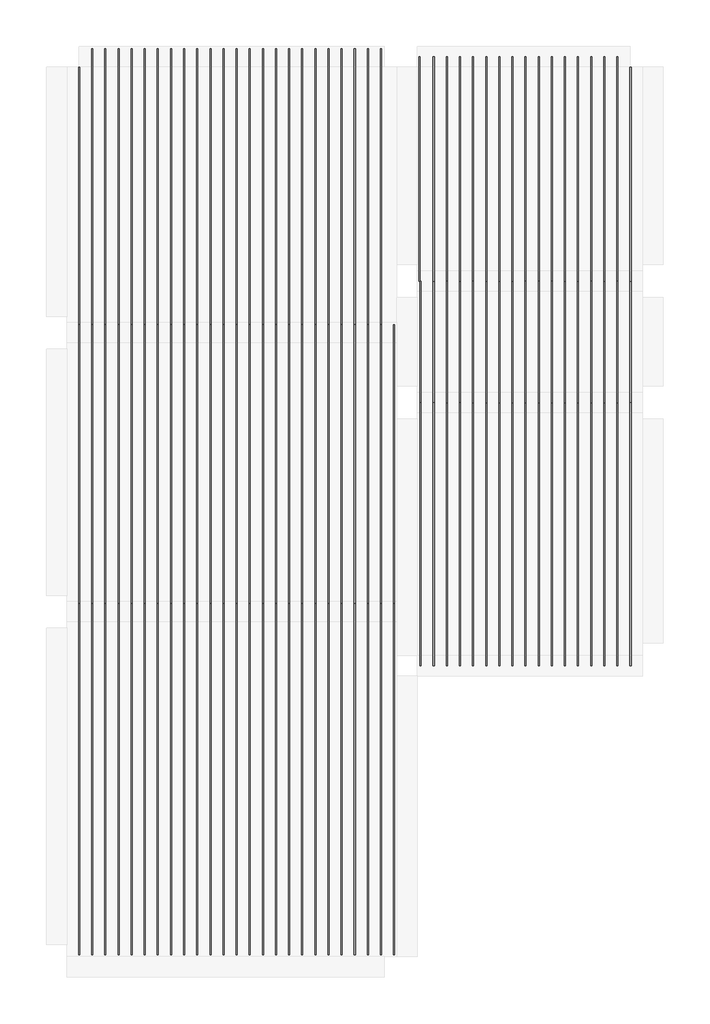
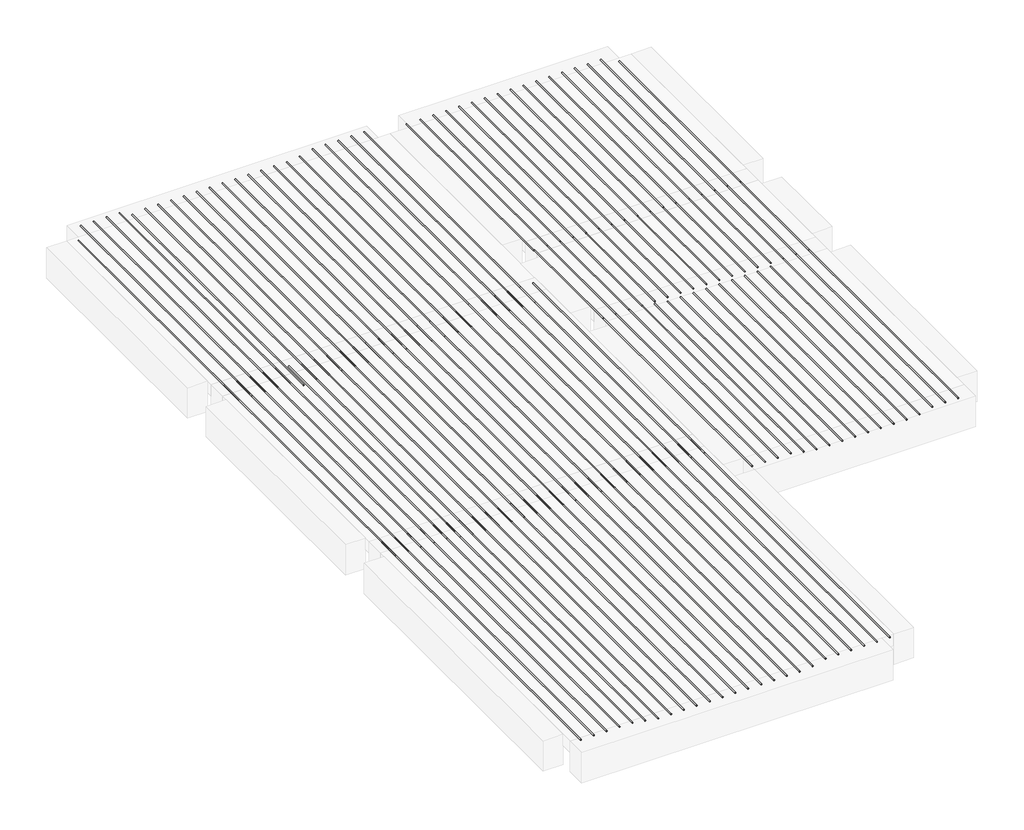
# One storey, part 2 of 2: 125 reinforcing bars.
"""IFC4 building model written with IfcOpenShell, lengths in millimetres."""

from ifc_helpers import new_model, si_unit, origin, place, context, project, spatial, polyline, segment, composite_curve, element, save
from ifc_brep_helpers import swept_disk

model = new_model("IFC4")

# Units and contexts
model_context = context("Model", 3, world=origin())
ifc_project = project(units=[si_unit("LENGTHUNIT", "METRE", prefix="MILLI")], contexts=[model_context])

# Site, building, storey
site = spatial("IfcSite", under=ifc_project)
building = spatial("IfcBuilding", under=site)
storey = spatial("IfcBuildingStorey", under=building, Elevation=0.0)

# Reinforcing bars
placement = place(None, origin())
element("IfcReinforcingBar", 1, at=placement, inside=storey, context=model_context, shape_type="SolidModel", body=[
    swept_disk(composite_curve([segment(polyline([(-8027.4883428, -144.0769256, -45.3573217), (-8027.4883428, 4206.4668244, -45.3573217)]), True, "CONTINUOUS")], self_intersect=False), 6.35),
])
element("IfcReinforcingBar", 2, at=placement, inside=storey, context=model_context, shape_type="SolidModel", body=[
    swept_disk(composite_curve([segment(polyline([(-8190.1883428, -144.0769256, -45.3573217), (-8190.1883428, 4206.4668244, -45.3573217)]), True, "CONTINUOUS")], self_intersect=False), 6.35),
])
element("IfcReinforcingBar", 3, at=placement, inside=storey, context=model_context, shape_type="SolidModel", body=[
    swept_disk(composite_curve([segment(polyline([(-8352.8883428, -144.0769256, -45.3573217), (-8352.8883428, 4206.4668244, -45.3573217)]), True, "CONTINUOUS")], self_intersect=False), 6.35),
])
element("IfcReinforcingBar", 4, at=placement, inside=storey, context=model_context, shape_type="SolidModel", body=[
    swept_disk(composite_curve([segment(polyline([(-8515.5883428, -144.0769256, -45.3573217), (-8515.5883428, 4206.4668244, -45.3573217)]), True, "CONTINUOUS")], self_intersect=False), 6.35),
])
element("IfcReinforcingBar", 5, at=placement, inside=storey, context=model_context, shape_type="SolidModel", body=[
    swept_disk(composite_curve([segment(polyline([(-8678.2883428, -144.0769256, -45.3573217), (-8678.2883428, 4206.4668244, -45.3573217)]), True, "CONTINUOUS")], self_intersect=False), 6.35),
])
element("IfcReinforcingBar", 6, at=placement, inside=storey, context=model_context, shape_type="SolidModel", body=[
    swept_disk(composite_curve([segment(polyline([(-8840.9883428, -144.0769256, -45.3573217), (-8840.9883428, 4206.4668244, -45.3573217)]), True, "CONTINUOUS")], self_intersect=False), 6.35),
])
element("IfcReinforcingBar", 7, at=placement, inside=storey, context=model_context, shape_type="SolidModel", body=[
    swept_disk(composite_curve([segment(polyline([(-9003.6883428, -144.0769256, -87.8573217), (-9003.6883428, 4206.4668244, -87.8573217)]), True, "CONTINUOUS")], self_intersect=False), 6.35),
])
element("IfcReinforcingBar", 8, at=placement, inside=storey, context=model_context, shape_type="SolidModel", body=[
    swept_disk(composite_curve([segment(polyline([(-11118.7883428, -144.0769256, -75.3573217), (-11118.7883428, 4206.4668244, -75.3573217)]), True, "CONTINUOUS")], self_intersect=False), 6.35),
])
element("IfcReinforcingBar", 9, at=placement, inside=storey, context=model_context, shape_type="SolidModel", body=[
    swept_disk(composite_curve([segment(polyline([(-11281.4883428, -144.0769256, -45.3573217), (-11281.4883428, 4206.4668244, -45.3573217)]), True, "CONTINUOUS")], self_intersect=False), 6.35),
])
element("IfcReinforcingBar", 10, at=placement, inside=storey, context=model_context, shape_type="SolidModel", body=[
    swept_disk(composite_curve([segment(polyline([(-11444.1883428, -144.0769256, -45.3573217), (-11444.1883428, 4206.4668244, -45.3573217)]), True, "CONTINUOUS")], self_intersect=False), 6.35),
])
element("IfcReinforcingBar", 11, at=placement, inside=storey, context=model_context, shape_type="SolidModel", body=[
    swept_disk(composite_curve([segment(polyline([(-11606.8883428, -144.0769256, -45.3573217), (-11606.8883428, 4206.4668244, -45.3573217)]), True, "CONTINUOUS")], self_intersect=False), 6.35),
])
element("IfcReinforcingBar", 12, at=placement, inside=storey, context=model_context, shape_type="SolidModel", body=[
    swept_disk(composite_curve([segment(polyline([(-11769.5883428, -144.0769256, -45.3573217), (-11769.5883428, 4206.4668244, -45.3573217)]), True, "CONTINUOUS")], self_intersect=False), 6.35),
])
element("IfcReinforcingBar", 13, at=placement, inside=storey, context=model_context, shape_type="SolidModel", body=[
    swept_disk(composite_curve([segment(polyline([(-11932.2883428, -144.0769256, -45.3573217), (-11932.2883428, 4206.4668244, -45.3573217)]), True, "CONTINUOUS")], self_intersect=False), 6.35),
])
element("IfcReinforcingBar", 14, at=placement, inside=storey, context=model_context, shape_type="SolidModel", body=[
    swept_disk(composite_curve([segment(polyline([(-9166.3883428, -144.0769256, -104.3861355), (-9166.3883428, 4206.4668244, -104.3861355)]), True, "CONTINUOUS")], self_intersect=False), 6.35),
])
element("IfcReinforcingBar", 15, at=placement, inside=storey, context=model_context, shape_type="SolidModel", body=[
    swept_disk(composite_curve([segment(polyline([(-9329.0883428, -144.0769256, -104.3861355), (-9329.0883428, 4206.4668244, -104.3861355)]), True, "CONTINUOUS")], self_intersect=False), 6.35),
])
element("IfcReinforcingBar", 16, at=placement, inside=storey, context=model_context, shape_type="SolidModel", body=[
    swept_disk(composite_curve([segment(polyline([(-9491.7883428, -144.0769256, -104.3861355), (-9491.7883428, 4206.4668244, -104.3861355)]), True, "CONTINUOUS")], self_intersect=False), 6.35),
])
element("IfcReinforcingBar", 17, at=placement, inside=storey, context=model_context, shape_type="SolidModel", body=[
    swept_disk(composite_curve([segment(polyline([(-9654.4883428, -144.0769256, -104.3861355), (-9654.4883428, 4206.4668244, -104.3861355)]), True, "CONTINUOUS")], self_intersect=False), 6.35),
])
element("IfcReinforcingBar", 18, at=placement, inside=storey, context=model_context, shape_type="SolidModel", body=[
    swept_disk(composite_curve([segment(polyline([(-9817.1883428, -144.0769256, -104.3861355), (-9817.1883428, 4206.4668244, -104.3861355)]), True, "CONTINUOUS")], self_intersect=False), 6.35),
])
element("IfcReinforcingBar", 19, at=placement, inside=storey, context=model_context, shape_type="SolidModel", body=[
    swept_disk(composite_curve([segment(polyline([(-9979.8883428, -144.0769256, -104.3861355), (-9979.8883428, 4206.4668244, -104.3861355)]), True, "CONTINUOUS")], self_intersect=False), 6.35),
])
element("IfcReinforcingBar", 20, at=placement, inside=storey, context=model_context, shape_type="SolidModel", body=[
    swept_disk(composite_curve([segment(polyline([(-10142.5883428, -144.0769256, -104.3861355), (-10142.5883428, 4206.4668244, -104.3861355)]), True, "CONTINUOUS")], self_intersect=False), 6.35),
])
element("IfcReinforcingBar", 21, at=placement, inside=storey, context=model_context, shape_type="SolidModel", body=[
    swept_disk(composite_curve([segment(polyline([(-10305.2883428, -144.0769256, -104.3861355), (-10305.2883428, 4206.4668244, -104.3861355)]), True, "CONTINUOUS")], self_intersect=False), 6.35),
])
element("IfcReinforcingBar", 22, at=placement, inside=storey, context=model_context, shape_type="SolidModel", body=[
    swept_disk(composite_curve([segment(polyline([(-10467.9883428, -144.0769256, -104.3861355), (-10467.9883428, 4206.4668244, -104.3861355)]), True, "CONTINUOUS")], self_intersect=False), 6.35),
])
element("IfcReinforcingBar", 23, at=placement, inside=storey, context=model_context, shape_type="SolidModel", body=[
    swept_disk(composite_curve([segment(polyline([(-10630.6883428, -144.0769256, -104.3861355), (-10630.6883428, 4206.4668244, -104.3861355)]), True, "CONTINUOUS")], self_intersect=False), 6.35),
])
element("IfcReinforcingBar", 24, at=placement, inside=storey, context=model_context, shape_type="SolidModel", body=[
    swept_disk(composite_curve([segment(polyline([(-10793.3883428, -144.0769256, -104.3861355), (-10793.3883428, 4206.4668244, -104.3861355)]), True, "CONTINUOUS")], self_intersect=False), 6.35),
])
element("IfcReinforcingBar", 25, at=placement, inside=storey, context=model_context, shape_type="SolidModel", body=[
    swept_disk(composite_curve([segment(polyline([(-10956.0883428, -144.0769256, -104.3861355), (-10956.0883428, 4206.4668244, -104.3861355)]), True, "CONTINUOUS")], self_intersect=False), 6.35),
])
element("IfcReinforcingBar", 26, at=placement, inside=storey, context=model_context, shape_type="SolidModel", body=[
    swept_disk(composite_curve([segment(polyline([(-8027.4883428, 3911.5030538, -45.3573217), (-8027.4883428, 7660.8668244, -45.3573217)]), True, "CONTINUOUS")], self_intersect=False), 6.35),
])
element("IfcReinforcingBar", 27, at=placement, inside=storey, context=model_context, shape_type="SolidModel", body=[
    swept_disk(composite_curve([segment(polyline([(-8190.1883428, 3911.5030538, -45.3573217), (-8190.1883428, 7660.8668244, -45.3573217)]), True, "CONTINUOUS")], self_intersect=False), 6.35),
])
element("IfcReinforcingBar", 28, at=placement, inside=storey, context=model_context, shape_type="SolidModel", body=[
    swept_disk(composite_curve([segment(polyline([(-8352.8883428, 3911.5030538, -45.3573217), (-8352.8883428, 7660.8668244, -45.3573217)]), True, "CONTINUOUS")], self_intersect=False), 6.35),
])
element("IfcReinforcingBar", 29, at=placement, inside=storey, context=model_context, shape_type="SolidModel", body=[
    swept_disk(composite_curve([segment(polyline([(-8515.5883428, 3911.5030538, -45.3573217), (-8515.5883428, 7660.8668244, -45.3573217)]), True, "CONTINUOUS")], self_intersect=False), 6.35),
])
element("IfcReinforcingBar", 30, at=placement, inside=storey, context=model_context, shape_type="SolidModel", body=[
    swept_disk(composite_curve([segment(polyline([(-8678.2883428, 3911.5030538, -45.3573217), (-8678.2883428, 7660.8668244, -45.3573217)]), True, "CONTINUOUS")], self_intersect=False), 6.35),
])
element("IfcReinforcingBar", 31, at=placement, inside=storey, context=model_context, shape_type="SolidModel", body=[
    swept_disk(composite_curve([segment(polyline([(-8840.9883428, 3911.5030538, -45.3573217), (-8840.9883428, 7660.8668244, -45.3573217)]), True, "CONTINUOUS")], self_intersect=False), 6.35),
])
element("IfcReinforcingBar", 32, at=placement, inside=storey, context=model_context, shape_type="SolidModel", body=[
    swept_disk(composite_curve([segment(polyline([(-9003.6883428, 3911.5030538, -87.8573217), (-9003.6883428, 7660.8668244, -87.8573217)]), True, "CONTINUOUS")], self_intersect=False), 6.35),
])
element("IfcReinforcingBar", 33, at=placement, inside=storey, context=model_context, shape_type="SolidModel", body=[
    swept_disk(composite_curve([segment(polyline([(-11118.7883428, 3911.5030538, -75.3573217), (-11118.7883428, 7660.8668244, -75.3573217)]), True, "CONTINUOUS")], self_intersect=False), 6.35),
])
element("IfcReinforcingBar", 34, at=placement, inside=storey, context=model_context, shape_type="SolidModel", body=[
    swept_disk(composite_curve([segment(polyline([(-11281.4883428, 3911.5030538, -45.3573217), (-11281.4883428, 7660.8668244, -45.3573217)]), True, "CONTINUOUS")], self_intersect=False), 6.35),
])
element("IfcReinforcingBar", 35, at=placement, inside=storey, context=model_context, shape_type="SolidModel", body=[
    swept_disk(composite_curve([segment(polyline([(-11444.1883428, 3911.5030538, -45.3573217), (-11444.1883428, 7660.8668244, -45.3573217)]), True, "CONTINUOUS")], self_intersect=False), 6.35),
])
element("IfcReinforcingBar", 36, at=placement, inside=storey, context=model_context, shape_type="SolidModel", body=[
    swept_disk(composite_curve([segment(polyline([(-11606.8883428, 3911.5030538, -45.3573217), (-11606.8883428, 7660.8668244, -45.3573217)]), True, "CONTINUOUS")], self_intersect=False), 6.35),
])
element("IfcReinforcingBar", 37, at=placement, inside=storey, context=model_context, shape_type="SolidModel", body=[
    swept_disk(composite_curve([segment(polyline([(-11769.5883428, 3911.5030538, -45.3573217), (-11769.5883428, 7660.8668244, -45.3573217)]), True, "CONTINUOUS")], self_intersect=False), 6.35),
])
element("IfcReinforcingBar", 38, at=placement, inside=storey, context=model_context, shape_type="SolidModel", body=[
    swept_disk(composite_curve([segment(polyline([(-11932.2883428, 3911.5030538, -45.3573217), (-11932.2883428, 7660.8668244, -45.3573217)]), True, "CONTINUOUS")], self_intersect=False), 6.35),
])
element("IfcReinforcingBar", 39, at=placement, inside=storey, context=model_context, shape_type="SolidModel", body=[
    swept_disk(composite_curve([segment(polyline([(-9166.3883428, 3911.5030538, -104.3861355), (-9166.3883428, 7660.8668244, -104.3861355)]), True, "CONTINUOUS")], self_intersect=False), 6.35),
])
element("IfcReinforcingBar", 40, at=placement, inside=storey, context=model_context, shape_type="SolidModel", body=[
    swept_disk(composite_curve([segment(polyline([(-9329.0883428, 3911.5030538, -104.3861355), (-9329.0883428, 7660.8668244, -104.3861355)]), True, "CONTINUOUS")], self_intersect=False), 6.35),
])
element("IfcReinforcingBar", 41, at=placement, inside=storey, context=model_context, shape_type="SolidModel", body=[
    swept_disk(composite_curve([segment(polyline([(-9491.7883428, 3911.5030538, -104.3861355), (-9491.7883428, 7660.8668244, -104.3861355)]), True, "CONTINUOUS")], self_intersect=False), 6.35),
])
element("IfcReinforcingBar", 42, at=placement, inside=storey, context=model_context, shape_type="SolidModel", body=[
    swept_disk(composite_curve([segment(polyline([(-9654.4883428, 3911.5030538, -104.3861355), (-9654.4883428, 7660.8668244, -104.3861355)]), True, "CONTINUOUS")], self_intersect=False), 6.35),
])
element("IfcReinforcingBar", 43, at=placement, inside=storey, context=model_context, shape_type="SolidModel", body=[
    swept_disk(composite_curve([segment(polyline([(-9817.1883428, 3911.5030538, -104.3861355), (-9817.1883428, 7660.8668244, -104.3861355)]), True, "CONTINUOUS")], self_intersect=False), 6.35),
])
element("IfcReinforcingBar", 44, at=placement, inside=storey, context=model_context, shape_type="SolidModel", body=[
    swept_disk(composite_curve([segment(polyline([(-9979.8883428, 3911.5030538, -104.3861355), (-9979.8883428, 7660.8668244, -104.3861355)]), True, "CONTINUOUS")], self_intersect=False), 6.35),
])
element("IfcReinforcingBar", 45, at=placement, inside=storey, context=model_context, shape_type="SolidModel", body=[
    swept_disk(composite_curve([segment(polyline([(-10142.5883428, 3911.5030538, -104.3861355), (-10142.5883428, 7660.8668244, -104.3861355)]), True, "CONTINUOUS")], self_intersect=False), 6.35),
])
element("IfcReinforcingBar", 46, at=placement, inside=storey, context=model_context, shape_type="SolidModel", body=[
    swept_disk(composite_curve([segment(polyline([(-10305.2883428, 3911.5030538, -104.3861355), (-10305.2883428, 7660.8668244, -104.3861355)]), True, "CONTINUOUS")], self_intersect=False), 6.35),
])
element("IfcReinforcingBar", 47, at=placement, inside=storey, context=model_context, shape_type="SolidModel", body=[
    swept_disk(composite_curve([segment(polyline([(-10467.9883428, 3911.5030538, -104.3861355), (-10467.9883428, 7660.8668244, -104.3861355)]), True, "CONTINUOUS")], self_intersect=False), 6.35),
])
element("IfcReinforcingBar", 48, at=placement, inside=storey, context=model_context, shape_type="SolidModel", body=[
    swept_disk(composite_curve([segment(polyline([(-10630.6883428, 3911.5030538, -104.3861355), (-10630.6883428, 7660.8668244, -104.3861355)]), True, "CONTINUOUS")], self_intersect=False), 6.35),
])
element("IfcReinforcingBar", 49, at=placement, inside=storey, context=model_context, shape_type="SolidModel", body=[
    swept_disk(composite_curve([segment(polyline([(-10793.3883428, 3911.5030538, -104.3861355), (-10793.3883428, 7660.8668244, -104.3861355)]), True, "CONTINUOUS")], self_intersect=False), 6.35),
])
element("IfcReinforcingBar", 50, at=placement, inside=storey, context=model_context, shape_type="SolidModel", body=[
    swept_disk(composite_curve([segment(polyline([(-10956.0883428, 3911.5030538, -104.3861355), (-10956.0883428, 7660.8668244, -104.3861355)]), True, "CONTINUOUS")], self_intersect=False), 6.35),
])
element("IfcReinforcingBar", 51, at=placement, inside=storey, context=model_context, shape_type="SolidModel", body=[
    swept_disk(composite_curve([segment(polyline([(-8190.1883428, 7334.1530538, -45.3573217), (-8190.1883428, 11083.5168244, -45.3573217)]), True, "CONTINUOUS")], self_intersect=False), 6.35),
])
element("IfcReinforcingBar", 52, at=placement, inside=storey, context=model_context, shape_type="SolidModel", body=[
    swept_disk(composite_curve([segment(polyline([(-8352.8883428, 7334.1530538, -45.3573217), (-8352.8883428, 11083.5168244, -45.3573217)]), True, "CONTINUOUS")], self_intersect=False), 6.35),
])
element("IfcReinforcingBar", 53, at=placement, inside=storey, context=model_context, shape_type="SolidModel", body=[
    swept_disk(composite_curve([segment(polyline([(-8515.5883428, 7334.1530538, -45.3573217), (-8515.5883428, 11083.5168244, -45.3573217)]), True, "CONTINUOUS")], self_intersect=False), 6.35),
])
element("IfcReinforcingBar", 54, at=placement, inside=storey, context=model_context, shape_type="SolidModel", body=[
    swept_disk(composite_curve([segment(polyline([(-8678.2883428, 7334.1530538, -45.3573217), (-8678.2883428, 11083.5168244, -45.3573217)]), True, "CONTINUOUS")], self_intersect=False), 6.35),
])
element("IfcReinforcingBar", 55, at=placement, inside=storey, context=model_context, shape_type="SolidModel", body=[
    swept_disk(composite_curve([segment(polyline([(-8840.9883428, 7334.1530538, -45.3573217), (-8840.9883428, 11083.5168244, -45.3573217)]), True, "CONTINUOUS")], self_intersect=False), 6.35),
])
element("IfcReinforcingBar", 56, at=placement, inside=storey, context=model_context, shape_type="SolidModel", body=[
    swept_disk(composite_curve([segment(polyline([(-9003.6883428, 7334.1530538, -87.8573217), (-9003.6883428, 11083.5168244, -87.8573217)]), True, "CONTINUOUS")], self_intersect=False), 6.35),
])
element("IfcReinforcingBar", 57, at=placement, inside=storey, context=model_context, shape_type="SolidModel", body=[
    swept_disk(composite_curve([segment(polyline([(-11118.7883428, 7334.1530538, -126.5541967), (-11118.7883428, 11083.5168244, -126.5541967)]), True, "CONTINUOUS")], self_intersect=False), 6.35),
])
element("IfcReinforcingBar", 58, at=placement, inside=storey, context=model_context, shape_type="SolidModel", body=[
    swept_disk(composite_curve([segment(polyline([(-11281.4883428, 7334.1530538, -45.3573217), (-11281.4883428, 11083.5168244, -45.3573217)]), True, "CONTINUOUS")], self_intersect=False), 6.35),
])
element("IfcReinforcingBar", 59, at=placement, inside=storey, context=model_context, shape_type="SolidModel", body=[
    swept_disk(composite_curve([segment(polyline([(-11444.1883428, 7334.1530538, -45.3573217), (-11444.1883428, 11083.5168244, -45.3573217)]), True, "CONTINUOUS")], self_intersect=False), 6.35),
])
element("IfcReinforcingBar", 60, at=placement, inside=storey, context=model_context, shape_type="SolidModel", body=[
    swept_disk(composite_curve([segment(polyline([(-11606.8883428, 7334.1530538, -45.3573217), (-11606.8883428, 11083.5168244, -45.3573217)]), True, "CONTINUOUS")], self_intersect=False), 6.35),
])
element("IfcReinforcingBar", 61, at=placement, inside=storey, context=model_context, shape_type="SolidModel", body=[
    swept_disk(composite_curve([segment(polyline([(-11769.5883428, 7334.1530538, -45.3573217), (-11769.5883428, 11083.5168244, -45.3573217)]), True, "CONTINUOUS")], self_intersect=False), 6.35),
])
element("IfcReinforcingBar", 62, at=placement, inside=storey, context=model_context, shape_type="SolidModel", body=[
    swept_disk(composite_curve([segment(polyline([(-11932.2883428, 7334.1530538, -45.3573217), (-11932.2883428, 10854.3967567, -45.3573217)]), True, "CONTINUOUS")], self_intersect=False), 6.35),
])
element("IfcReinforcingBar", 63, at=placement, inside=storey, context=model_context, shape_type="SolidModel", body=[
    swept_disk(composite_curve([segment(polyline([(-9166.3883428, 7334.1530538, -104.3861355), (-9166.3883428, 11083.5168244, -104.3861355)]), True, "CONTINUOUS")], self_intersect=False), 6.35),
])
element("IfcReinforcingBar", 64, at=placement, inside=storey, context=model_context, shape_type="SolidModel", body=[
    swept_disk(composite_curve([segment(polyline([(-9329.0883428, 7334.1530538, -104.3861355), (-9329.0883428, 11083.5168244, -104.3861355)]), True, "CONTINUOUS")], self_intersect=False), 6.35),
])
element("IfcReinforcingBar", 65, at=placement, inside=storey, context=model_context, shape_type="SolidModel", body=[
    swept_disk(composite_curve([segment(polyline([(-9491.7883428, 7334.1530538, -104.3861355), (-9491.7883428, 11083.5168244, -104.3861355)]), True, "CONTINUOUS")], self_intersect=False), 6.35),
])
element("IfcReinforcingBar", 66, at=placement, inside=storey, context=model_context, shape_type="SolidModel", body=[
    swept_disk(composite_curve([segment(polyline([(-9654.4883428, 7334.1530538, -104.3861355), (-9654.4883428, 11083.5168244, -104.3861355)]), True, "CONTINUOUS")], self_intersect=False), 6.35),
])
element("IfcReinforcingBar", 67, at=placement, inside=storey, context=model_context, shape_type="SolidModel", body=[
    swept_disk(composite_curve([segment(polyline([(-9817.1883428, 7334.1530538, -104.3861355), (-9817.1883428, 11083.5168244, -104.3861355)]), True, "CONTINUOUS")], self_intersect=False), 6.35),
])
element("IfcReinforcingBar", 68, at=placement, inside=storey, context=model_context, shape_type="SolidModel", body=[
    swept_disk(composite_curve([segment(polyline([(-9979.8883428, 7334.1530538, -104.3861355), (-9979.8883428, 11083.5168244, -104.3861355)]), True, "CONTINUOUS")], self_intersect=False), 6.35),
])
element("IfcReinforcingBar", 69, at=placement, inside=storey, context=model_context, shape_type="SolidModel", body=[
    swept_disk(composite_curve([segment(polyline([(-10142.5883428, 7334.1530538, -104.3861355), (-10142.5883428, 11083.5168244, -104.3861355)]), True, "CONTINUOUS")], self_intersect=False), 6.35),
])
element("IfcReinforcingBar", 70, at=placement, inside=storey, context=model_context, shape_type="SolidModel", body=[
    swept_disk(composite_curve([segment(polyline([(-10305.2883428, 7334.1530538, -104.3861355), (-10305.2883428, 11083.5168244, -104.3861355)]), True, "CONTINUOUS")], self_intersect=False), 6.35),
])
element("IfcReinforcingBar", 71, at=placement, inside=storey, context=model_context, shape_type="SolidModel", body=[
    swept_disk(composite_curve([segment(polyline([(-10467.9883428, 7334.1530538, -104.3861355), (-10467.9883428, 11083.5168244, -104.3861355)]), True, "CONTINUOUS")], self_intersect=False), 6.35),
])
element("IfcReinforcingBar", 72, at=placement, inside=storey, context=model_context, shape_type="SolidModel", body=[
    swept_disk(composite_curve([segment(polyline([(-10630.6883428, 7334.1530538, -104.3861355), (-10630.6883428, 11083.5168244, -104.3861355)]), True, "CONTINUOUS")], self_intersect=False), 6.35),
])
element("IfcReinforcingBar", 73, at=placement, inside=storey, context=model_context, shape_type="SolidModel", body=[
    swept_disk(composite_curve([segment(polyline([(-10793.3883428, 7334.1530538, -104.3861355), (-10793.3883428, 11083.5168244, -104.3861355)]), True, "CONTINUOUS")], self_intersect=False), 6.35),
])
element("IfcReinforcingBar", 74, at=placement, inside=storey, context=model_context, shape_type="SolidModel", body=[
    swept_disk(composite_curve([segment(polyline([(-10956.0883428, 7334.1530538, -104.3861355), (-10956.0883428, 11083.5168244, -104.3861355)]), True, "CONTINUOUS")], self_intersect=False), 6.35),
])
element("IfcReinforcingBar", 75, at=placement, inside=storey, context=model_context, shape_type="SolidModel", body=[
    swept_disk(composite_curve([segment(polyline([(-7699.7883428, 3437.7199494, -45.3573217), (-7699.7883428, 6695.2699494, -45.3573217)]), True, "CONTINUOUS")], self_intersect=False), 6.35),
])
element("IfcReinforcingBar", 76, at=placement, inside=storey, context=model_context, shape_type="SolidModel", body=[
    swept_disk(composite_curve([segment(polyline([(-7537.0883428, 3437.7199494, -45.3573217), (-7537.0883428, 6695.2699494, -45.3573217)]), True, "CONTINUOUS")], self_intersect=False), 6.35),
])
element("IfcReinforcingBar", 77, at=placement, inside=storey, context=model_context, shape_type="SolidModel", body=[
    swept_disk(composite_curve([segment(polyline([(-7374.3883428, 3437.7199494, -45.3573217), (-7374.3883428, 6695.2699494, -45.3573217)]), True, "CONTINUOUS")], self_intersect=False), 6.35),
])
element("IfcReinforcingBar", 78, at=placement, inside=storey, context=model_context, shape_type="SolidModel", body=[
    swept_disk(composite_curve([segment(polyline([(-7211.6883428, 3437.7199494, -45.3573217), (-7211.6883428, 6695.2699494, -45.3573217)]), True, "CONTINUOUS")], self_intersect=False), 6.35),
])
element("IfcReinforcingBar", 79, at=placement, inside=storey, context=model_context, shape_type="SolidModel", body=[
    swept_disk(composite_curve([segment(polyline([(-7048.9883428, 3437.7199494, -77.8573217), (-7048.9883428, 6695.2699494, -77.8573217)]), True, "CONTINUOUS")], self_intersect=False), 6.35),
])
element("IfcReinforcingBar", 80, at=placement, inside=storey, context=model_context, shape_type="SolidModel", body=[
    swept_disk(composite_curve([segment(polyline([(-6886.2883428, 3437.7199494, -104.7323217), (-6886.2883428, 6695.2699494, -104.7323217)]), True, "CONTINUOUS")], self_intersect=False), 6.35),
])
element("IfcReinforcingBar", 81, at=placement, inside=storey, context=model_context, shape_type="SolidModel", body=[
    swept_disk(composite_curve([segment(polyline([(-6723.5883428, 3437.7199494, -104.7323217), (-6723.5883428, 6695.2699494, -104.7323217)]), True, "CONTINUOUS")], self_intersect=False), 6.35),
])
element("IfcReinforcingBar", 82, at=placement, inside=storey, context=model_context, shape_type="SolidModel", body=[
    swept_disk(composite_curve([segment(polyline([(-6560.8883428, 3437.7199494, -104.7323217), (-6560.8883428, 6695.2699494, -104.7323217)]), True, "CONTINUOUS")], self_intersect=False), 6.35),
])
element("IfcReinforcingBar", 83, at=placement, inside=storey, context=model_context, shape_type="SolidModel", body=[
    swept_disk(composite_curve([segment(polyline([(-6398.1883428, 3437.7199494, -104.7323217), (-6398.1883428, 6695.2699494, -104.7323217)]), True, "CONTINUOUS")], self_intersect=False), 6.35),
])
element("IfcReinforcingBar", 84, at=placement, inside=storey, context=model_context, shape_type="SolidModel", body=[
    swept_disk(composite_curve([segment(polyline([(-6235.4883428, 3437.7199494, -104.7323217), (-6235.4883428, 6695.2699494, -104.7323217)]), True, "CONTINUOUS")], self_intersect=False), 6.35),
])
element("IfcReinforcingBar", 85, at=placement, inside=storey, context=model_context, shape_type="SolidModel", body=[
    swept_disk(composite_curve([segment(polyline([(-6072.7883428, 3437.7199494, -104.7323217), (-6072.7883428, 6695.2699494, -104.7323217)]), True, "CONTINUOUS")], self_intersect=False), 6.35),
])
element("IfcReinforcingBar", 86, at=placement, inside=storey, context=model_context, shape_type="SolidModel", body=[
    swept_disk(composite_curve([segment(polyline([(-5910.0883428, 3437.7199494, -104.7323217), (-5910.0883428, 6695.2699494, -104.7323217)]), True, "CONTINUOUS")], self_intersect=False), 6.35),
])
element("IfcReinforcingBar", 87, at=placement, inside=storey, context=model_context, shape_type="SolidModel", body=[
    swept_disk(composite_curve([segment(polyline([(-5747.3883428, 3437.7199494, -104.7323217), (-5747.3883428, 6695.2699494, -104.7323217)]), True, "CONTINUOUS")], self_intersect=False), 6.35),
])
element("IfcReinforcingBar", 88, at=placement, inside=storey, context=model_context, shape_type="SolidModel", body=[
    swept_disk(composite_curve([segment(polyline([(-5584.6883428, 3437.7199494, -93.1698217), (-5584.6883428, 6695.2699494, -93.1698217)]), True, "CONTINUOUS")], self_intersect=False), 6.35),
])
element("IfcReinforcingBar", 89, at=placement, inside=storey, context=model_context, shape_type="SolidModel", body=[
    swept_disk(composite_curve([segment(polyline([(-5421.9883428, 3437.7199494, -49.1073217), (-5421.9883428, 6695.2699494, -49.1073217)]), True, "CONTINUOUS")], self_intersect=False), 6.35),
])
element("IfcReinforcingBar", 90, at=placement, inside=storey, context=model_context, shape_type="SolidModel", body=[
    swept_disk(composite_curve([segment(polyline([(-5259.2883428, 3437.7199494, -45.3573217), (-5259.2883428, 6695.2699494, -45.3573217)]), True, "CONTINUOUS")], self_intersect=False), 6.35),
])
element("IfcReinforcingBar", 91, at=placement, inside=storey, context=model_context, shape_type="SolidModel", body=[
    swept_disk(composite_curve([segment(polyline([(-5096.5883428, 3437.7199494, -45.3573217), (-5096.5883428, 6695.2699494, -45.3573217)]), True, "CONTINUOUS")], self_intersect=False), 6.35),
])
element("IfcReinforcingBar", 92, at=placement, inside=storey, context=model_context, shape_type="SolidModel", body=[
    swept_disk(composite_curve([segment(polyline([(-7699.7883428, 6695.2699494, -45.3573217), (-7699.7883428, 8200.2199494, -45.3573217)]), True, "CONTINUOUS")], self_intersect=False), 6.35),
])
element("IfcReinforcingBar", 93, at=placement, inside=storey, context=model_context, shape_type="SolidModel", body=[
    swept_disk(composite_curve([segment(polyline([(-7537.0883428, 6695.2699494, -45.3573217), (-7537.0883428, 8200.2199494, -45.3573217)]), True, "CONTINUOUS")], self_intersect=False), 6.35),
])
element("IfcReinforcingBar", 94, at=placement, inside=storey, context=model_context, shape_type="SolidModel", body=[
    swept_disk(composite_curve([segment(polyline([(-7374.3883428, 6695.2699494, -45.3573217), (-7374.3883428, 8200.2199494, -45.3573217)]), True, "CONTINUOUS")], self_intersect=False), 6.35),
])
element("IfcReinforcingBar", 95, at=placement, inside=storey, context=model_context, shape_type="SolidModel", body=[
    swept_disk(composite_curve([segment(polyline([(-7211.6883428, 6695.2699494, -45.3573217), (-7211.6883428, 8200.2199494, -45.3573217)]), True, "CONTINUOUS")], self_intersect=False), 6.35),
])
element("IfcReinforcingBar", 96, at=placement, inside=storey, context=model_context, shape_type="SolidModel", body=[
    swept_disk(composite_curve([segment(polyline([(-7048.9883428, 6695.2699494, -45.3573217), (-7048.9883428, 8200.2199494, -45.3573217)]), True, "CONTINUOUS")], self_intersect=False), 6.35),
])
element("IfcReinforcingBar", 97, at=placement, inside=storey, context=model_context, shape_type="SolidModel", body=[
    swept_disk(composite_curve([segment(polyline([(-6886.2883428, 6695.2699494, -45.3573217), (-6886.2883428, 8200.2199494, -45.3573217)]), True, "CONTINUOUS")], self_intersect=False), 6.35),
])
element("IfcReinforcingBar", 98, at=placement, inside=storey, context=model_context, shape_type="SolidModel", body=[
    swept_disk(composite_curve([segment(polyline([(-6723.5883428, 6695.2699494, -45.3573217), (-6723.5883428, 8200.2199494, -45.3573217)]), True, "CONTINUOUS")], self_intersect=False), 6.35),
])
element("IfcReinforcingBar", 99, at=placement, inside=storey, context=model_context, shape_type="SolidModel", body=[
    swept_disk(composite_curve([segment(polyline([(-6560.8883428, 6695.2699494, -45.3573217), (-6560.8883428, 8200.2199494, -45.3573217)]), True, "CONTINUOUS")], self_intersect=False), 6.35),
])
element("IfcReinforcingBar", 100, at=placement, inside=storey, context=model_context, shape_type="SolidModel", body=[
    swept_disk(composite_curve([segment(polyline([(-6398.1883428, 6695.2699494, -45.3573217), (-6398.1883428, 8200.2199494, -45.3573217)]), True, "CONTINUOUS")], self_intersect=False), 6.35),
])
element("IfcReinforcingBar", 101, at=placement, inside=storey, context=model_context, shape_type="SolidModel", body=[
    swept_disk(composite_curve([segment(polyline([(-6235.4883428, 6695.2699494, -45.3573217), (-6235.4883428, 8200.2199494, -45.3573217)]), True, "CONTINUOUS")], self_intersect=False), 6.35),
])
element("IfcReinforcingBar", 102, at=placement, inside=storey, context=model_context, shape_type="SolidModel", body=[
    swept_disk(composite_curve([segment(polyline([(-6072.7883428, 6695.2699494, -45.3573217), (-6072.7883428, 8200.2199494, -45.3573217)]), True, "CONTINUOUS")], self_intersect=False), 6.35),
])
element("IfcReinforcingBar", 103, at=placement, inside=storey, context=model_context, shape_type="SolidModel", body=[
    swept_disk(composite_curve([segment(polyline([(-5910.0883428, 6695.2699494, -45.3573217), (-5910.0883428, 8200.2199494, -45.3573217)]), True, "CONTINUOUS")], self_intersect=False), 6.35),
])
element("IfcReinforcingBar", 104, at=placement, inside=storey, context=model_context, shape_type="SolidModel", body=[
    swept_disk(composite_curve([segment(polyline([(-5747.3883428, 6695.2699494, -45.3573217), (-5747.3883428, 8200.2199494, -45.3573217)]), True, "CONTINUOUS")], self_intersect=False), 6.35),
])
element("IfcReinforcingBar", 105, at=placement, inside=storey, context=model_context, shape_type="SolidModel", body=[
    swept_disk(composite_curve([segment(polyline([(-5584.6883428, 6695.2699494, -45.3573217), (-5584.6883428, 8200.2199494, -45.3573217)]), True, "CONTINUOUS")], self_intersect=False), 6.35),
])
element("IfcReinforcingBar", 106, at=placement, inside=storey, context=model_context, shape_type="SolidModel", body=[
    swept_disk(composite_curve([segment(polyline([(-5421.9883428, 6695.2699494, -45.3573217), (-5421.9883428, 8200.2199494, -45.3573217)]), True, "CONTINUOUS")], self_intersect=False), 6.35),
])
element("IfcReinforcingBar", 107, at=placement, inside=storey, context=model_context, shape_type="SolidModel", body=[
    swept_disk(composite_curve([segment(polyline([(-5259.2883428, 6695.2699494, -45.3573217), (-5259.2883428, 8200.2199494, -45.3573217)]), True, "CONTINUOUS")], self_intersect=False), 6.35),
])
element("IfcReinforcingBar", 108, at=placement, inside=storey, context=model_context, shape_type="SolidModel", body=[
    swept_disk(composite_curve([segment(polyline([(-5096.5883428, 6695.2699494, -45.3573217), (-5096.5883428, 8200.2199494, -45.3573217)]), True, "CONTINUOUS")], self_intersect=False), 6.35),
])
element("IfcReinforcingBar", 109, at=placement, inside=storey, context=model_context, shape_type="SolidModel", body=[
    swept_disk(composite_curve([segment(polyline([(-5096.5883428, 8200.2199494, -45.3573217), (-5096.5883428, 10854.4524966, -45.3573217)]), True, "CONTINUOUS")], self_intersect=False), 6.35),
])
element("IfcReinforcingBar", 110, at=placement, inside=storey, context=model_context, shape_type="SolidModel", body=[
    swept_disk(composite_curve([segment(polyline([(-5259.2883428, 8200.2199494, -45.3573217), (-5259.2883428, 10981.5199494, -45.3573217)]), True, "CONTINUOUS")], self_intersect=False), 6.35),
])
element("IfcReinforcingBar", 111, at=placement, inside=storey, context=model_context, shape_type="SolidModel", body=[
    swept_disk(composite_curve([segment(polyline([(-5421.9883428, 8200.2199494, -45.3573217), (-5421.9883428, 10981.5199494, -45.3573217)]), True, "CONTINUOUS")], self_intersect=False), 6.35),
])
element("IfcReinforcingBar", 112, at=placement, inside=storey, context=model_context, shape_type="SolidModel", body=[
    swept_disk(composite_curve([segment(polyline([(-5584.6883428, 8200.2199494, -45.3573217), (-5584.6883428, 10981.5199494, -45.3573217)]), True, "CONTINUOUS")], self_intersect=False), 6.35),
])
element("IfcReinforcingBar", 113, at=placement, inside=storey, context=model_context, shape_type="SolidModel", body=[
    swept_disk(composite_curve([segment(polyline([(-5747.3883428, 8200.2199494, -45.3573217), (-5747.3883428, 10981.5199494, -45.3573217)]), True, "CONTINUOUS")], self_intersect=False), 6.35),
])
element("IfcReinforcingBar", 114, at=placement, inside=storey, context=model_context, shape_type="SolidModel", body=[
    swept_disk(composite_curve([segment(polyline([(-5910.0883428, 8200.2199494, -45.3573217), (-5910.0883428, 10981.5199494, -45.3573217)]), True, "CONTINUOUS")], self_intersect=False), 6.35),
])
element("IfcReinforcingBar", 115, at=placement, inside=storey, context=model_context, shape_type="SolidModel", body=[
    swept_disk(composite_curve([segment(polyline([(-6072.7883428, 8200.2199494, -45.3573217), (-6072.7883428, 10981.5199494, -45.3573217)]), True, "CONTINUOUS")], self_intersect=False), 6.35),
])
element("IfcReinforcingBar", 116, at=placement, inside=storey, context=model_context, shape_type="SolidModel", body=[
    swept_disk(composite_curve([segment(polyline([(-6235.4883428, 8200.2199494, -45.3573217), (-6235.4883428, 10981.5199494, -45.3573217)]), True, "CONTINUOUS")], self_intersect=False), 6.35),
])
element("IfcReinforcingBar", 117, at=placement, inside=storey, context=model_context, shape_type="SolidModel", body=[
    swept_disk(composite_curve([segment(polyline([(-6398.1883428, 8200.2199494, -45.3573217), (-6398.1883428, 10981.5199494, -45.3573217)]), True, "CONTINUOUS")], self_intersect=False), 6.35),
])
element("IfcReinforcingBar", 118, at=placement, inside=storey, context=model_context, shape_type="SolidModel", body=[
    swept_disk(composite_curve([segment(polyline([(-6560.8883428, 8200.2199494, -45.3573217), (-6560.8883428, 10981.5199494, -45.3573217)]), True, "CONTINUOUS")], self_intersect=False), 6.35),
])
element("IfcReinforcingBar", 119, at=placement, inside=storey, context=model_context, shape_type="SolidModel", body=[
    swept_disk(composite_curve([segment(polyline([(-6723.5883428, 8200.2199494, -45.3573217), (-6723.5883428, 10981.5199494, -45.3573217)]), True, "CONTINUOUS")], self_intersect=False), 6.35),
])
element("IfcReinforcingBar", 120, at=placement, inside=storey, context=model_context, shape_type="SolidModel", body=[
    swept_disk(composite_curve([segment(polyline([(-6886.2883428, 8200.2199494, -45.3573217), (-6886.2883428, 10981.5199494, -45.3573217)]), True, "CONTINUOUS")], self_intersect=False), 6.35),
])
element("IfcReinforcingBar", 121, at=placement, inside=storey, context=model_context, shape_type="SolidModel", body=[
    swept_disk(composite_curve([segment(polyline([(-7048.9883428, 8200.2199494, -45.3573217), (-7048.9883428, 10981.5199494, -45.3573217)]), True, "CONTINUOUS")], self_intersect=False), 6.35),
])
element("IfcReinforcingBar", 122, at=placement, inside=storey, context=model_context, shape_type="SolidModel", body=[
    swept_disk(composite_curve([segment(polyline([(-7211.6883428, 8200.2199494, -45.3573217), (-7211.6883428, 10981.5199494, -45.3573217)]), True, "CONTINUOUS")], self_intersect=False), 6.35),
])
element("IfcReinforcingBar", 123, at=placement, inside=storey, context=model_context, shape_type="SolidModel", body=[
    swept_disk(composite_curve([segment(polyline([(-7374.3883428, 8200.2199494, -45.3573217), (-7374.3883428, 10981.5199494, -45.3573217)]), True, "CONTINUOUS")], self_intersect=False), 6.35),
])
element("IfcReinforcingBar", 124, at=placement, inside=storey, context=model_context, shape_type="SolidModel", body=[
    swept_disk(composite_curve([segment(polyline([(-7537.0883428, 8200.2199494, -45.3573217), (-7537.0883428, 10981.5199494, -45.3573217)]), True, "CONTINUOUS")], self_intersect=False), 6.35),
])
element("IfcReinforcingBar", 125, at=placement, inside=storey, context=model_context, shape_type="SolidModel", body=[
    swept_disk(composite_curve([segment(polyline([(-7712.8852178, 8200.2199494, -45.3573217), (-7712.8852178, 10981.5199494, -45.3573217)]), True, "CONTINUOUS")], self_intersect=False), 6.35),
])

save(model, "model.ifc")

# Revit data of these elements
# Elements 1, 2, 3, 4, 5, 6, 7, 8, 9, 10, 11, 12, 13, 14, 15, 16, 17, 18, 19, 20, 21, 22, 23, 24, 25, 26, 27, 28, 29, 30, 31, 32, 33, 34, 35, 36, 37, 38, 39, 40, 41, 42, 43, 44, 45, 46, 47, 48, 49, 50, 51, 52, 53, 54, 55, 56, 57, 58, 59, 60, 61, 62, 63, 64, 65, 66, 67, 68, 69, 70, 71, 72, 73, 74, 75, 76, 77, 78, 79, 80, 81, 82, 83, 84, 85, 86, 87, 88, 89, 90, 91, 92, 93, 94, 95, 96, 97, 98, 99, 100, 101, 102, 103, 104, 105, 106, 107, 108, 109, 110, 111, 112, 113, 114, 115, 116, 117, 118, 119, 120, 121, 122, 123, 124, 125 (IfcReinforcingBar)
#   Phase Created = New Construction
